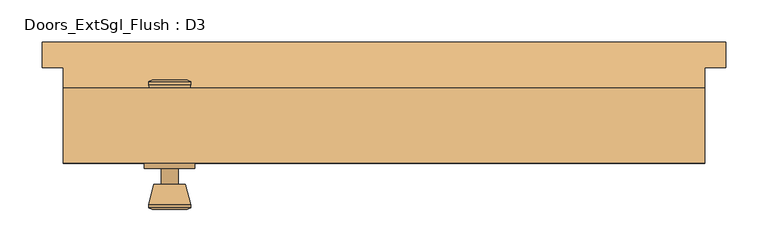
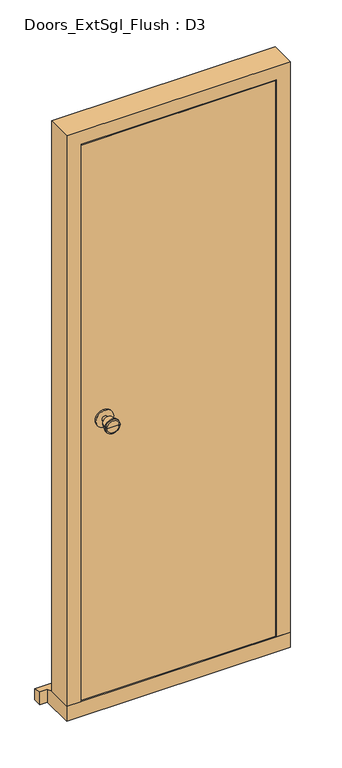
"""IFC4 building model written with IfcOpenShell, lengths in millimetres: door geometry, Doors_ExtSgl_Flush : D3."""

from ifc_helpers import new_model, si_unit, point, frame, frame_2d, origin, place, context, project, spatial, polyline, circle_curve, trimmed, segment, composite_curve, outline, extrude, faceted_brep, source, transform, mapped, element, save
from ifc_brep_helpers import plane_surface, cylinder_surface, revolved_surface, advanced_brep


def doors_extsgl_flush_d3_fcdd24de(model_context):
    return source(origin(), model_context, "Body", "SolidModel", [
        advanced_brep(
        [(-254.5, -85.1004, 1050.0), (-244.5, -85.1004, 1050.0), (-264.5, -85.1004, 1050.0), (-234.0241324, -134.1004, 1050.0), (-254.5, -134.1004, 1050.0), (-274.9758676, -134.1004, 1050.0), (-229.5, -132.2725319, 1050.0), (-279.5, -132.2725319, 1050.0), (-229.5, -128.8088537, 1050.0), (-279.5, -128.8088537, 1050.0), (-235.863764, -104.1004, 1050.0), (-273.136236, -104.1004, 1050.0), (-244.5, -104.1004, 1050.0), (-264.5, -104.1004, 1050.0)],
        [
            (0, 1),
            (1, 2, circle_curve(frame((-254.5, -85.1004, 1050.0), z_axis=(0.0, 1.0, 0.0), x_axis=(-1.0, 0.0, 0.0)), 10.0)),
            (2, 0),
            (2, 1, circle_curve(frame((-254.5, -85.1004, 1050.0), z_axis=(0.0, 1.0, 0.0), x_axis=(-1.0, 0.0, 0.0)), 10.0)),
            (3, 4),
            (4, 5),
            (5, 3, circle_curve(frame((-254.5, -134.1004, 1050.0), z_axis=(0.0, -1.0, 0.0), x_axis=(-1.0, 0.0, 0.0)), 20.4758676)),
            (3, 5, circle_curve(frame((-254.5, -134.1004, 1050.0), z_axis=(0.0, -1.0, 0.0), x_axis=(-1.0, 0.0, 0.0)), 20.4758676)),
            (6, 3),
            (5, 7),
            (7, 6, circle_curve(frame((-254.5, -132.2725319, 1050.0), z_axis=(0.0, -1.0, 0.0), x_axis=(-1.0, 0.0, 0.0)), 25.0)),
            (6, 7, circle_curve(frame((-254.5, -132.2725319, 1050.0), z_axis=(0.0, -1.0, 0.0), x_axis=(-1.0, 0.0, 0.0)), 25.0)),
            (8, 6),
            (7, 9),
            (9, 8, circle_curve(frame((-254.5, -128.8088537, 1050.0), z_axis=(0.0, -1.0, 0.0), x_axis=(-1.0, 0.0, 0.0)), 25.0)),
            (8, 9, circle_curve(frame((-254.5, -128.8088537, 1050.0), z_axis=(0.0, -1.0, 0.0), x_axis=(-1.0, 0.0, 0.0)), 25.0)),
            (10, 8),
            (9, 11),
            (11, 10, circle_curve(frame((-254.5, -104.1004, 1050.0), z_axis=(0.0, -1.0, 0.0), x_axis=(-1.0, 0.0, 0.0)), 18.636236)),
            (10, 11, circle_curve(frame((-254.5, -104.1004, 1050.0), z_axis=(0.0, -1.0, 0.0), x_axis=(-1.0, 0.0, 0.0)), 18.636236)),
            (12, 10),
            (11, 13),
            (13, 12, circle_curve(frame((-254.5, -104.1004, 1050.0), z_axis=(0.0, -1.0, 0.0), x_axis=(-1.0, 0.0, 0.0)), 10.0)),
            (12, 13, circle_curve(frame((-254.5, -104.1004, 1050.0), z_axis=(0.0, -1.0, 0.0), x_axis=(-1.0, 0.0, 0.0)), 10.0)),
            (1, 12),
            (13, 2),
        ],
        [
            plane_surface(frame((-254.5, -85.1004, 1050.0), z_axis=(0.0, 1.0, 0.0), x_axis=(-1.0, 0.0, 0.0))),
            plane_surface(frame((-254.5, -134.1004, 1050.0), z_axis=(0.0, -1.0, 0.0), x_axis=(-1.0, 0.0, 0.0))),
            revolved_surface(polyline([(-274.9758676, -134.1004, 1050.0), (-279.5, -132.2725319, 1050.0)]), (-254.5, -85.1004, 1050.0), (0.0, 1.0, 0.0)),
            cylinder_surface(frame((-254.5, -85.1004, 1050.0), z_axis=(0.0, 1.0, 0.0), x_axis=(-1.0, 0.0, 0.0)), 25.0),
            revolved_surface(polyline([(-279.5, -128.8088537, 1050.0), (-273.136236, -104.1004, 1050.0)]), (-254.5, -85.1004, 1050.0), (0.0, 1.0, 0.0)),
            plane_surface(frame((-254.5, -104.1004, 1050.0), z_axis=(0.0, 1.0, 0.0), x_axis=(-1.0, 0.0, 0.0))),
            cylinder_surface(frame((-254.5, -85.1004, 1050.0), z_axis=(0.0, 1.0, 0.0), x_axis=(-1.0, 0.0, 0.0)), 10.0),
        ],
        [
            (0, [[1, 2, 3]]),
            (0, [[-3, 4, -1]]),
            (1, [[5, 6, 7]]),
            (1, [[-6, -5, 8]]),
            (2, [[9, -7, 10, 11]]),
            (2, [[-10, -8, -9, 12]]),
            (3, [[13, -11, 14, 15]]),
            (3, [[-14, -12, -13, 16]]),
            (4, [[17, -15, 18, 19]]),
            (4, [[-18, -16, -17, 20]]),
            (5, [[21, -19, 22, 23]]),
            (5, [[-22, -20, -21, 24]]),
            (6, [[25, -23, 26, -2]]),
            (6, [[-26, -24, -25, -4]]),
        ],
    ),
        extrude(outline(composite_curve([segment(trimmed(circle_curve(frame_2d((1050.0, -254.5)), 30.0), [point((1050.0, -284.5))], [point((1050.0, -224.5))], False, "CARTESIAN"), True, "CONTINUOUS"), segment(trimmed(circle_curve(frame_2d((1050.0, -254.5)), 30.0), [point((1050.0, -224.5))], [point((1050.0, -284.5))], False, "CARTESIAN"), True, "CONTINUOUS")], self_intersect=False)), frame((0.0, -85.1004, 0.0), z_axis=(0.0, 1.0, 0.0), x_axis=(0.0, 0.0, 1.0)), (0.0, 0.0, 1.0), 6.0),
        advanced_brep(
        [(-254.5, -29.1004, 1050.0), (-264.5, -29.1004, 1050.0), (-244.5, -29.1004, 1050.0), (-234.0241324, 19.8996, 1050.0), (-274.9758676, 19.8996, 1050.0), (-254.5, 19.8996, 1050.0), (-229.5, 18.0717319, 1050.0), (-279.5, 18.0717319, 1050.0), (-229.5, 14.6080537, 1050.0), (-279.5, 14.6080537, 1050.0), (-235.863764, -10.1004, 1050.0), (-273.136236, -10.1004, 1050.0), (-244.5, -10.1004, 1050.0), (-264.5, -10.1004, 1050.0)],
        [
            (0, 1),
            (1, 2, circle_curve(frame((-254.5, -29.1004, 1050.0), z_axis=(0.0, -1.0, 0.0), x_axis=(-1.0, 0.0, 0.0)), 10.0)),
            (2, 0),
            (2, 1, circle_curve(frame((-254.5, -29.1004, 1050.0), z_axis=(0.0, -1.0, 0.0), x_axis=(-1.0, 0.0, 0.0)), 10.0)),
            (3, 4, circle_curve(frame((-254.5, 19.8996, 1050.0), z_axis=(0.0, 1.0, 0.0), x_axis=(-1.0, 0.0, 0.0)), 20.4758676)),
            (4, 5),
            (5, 3),
            (4, 3, circle_curve(frame((-254.5, 19.8996, 1050.0), z_axis=(0.0, 1.0, 0.0), x_axis=(-1.0, 0.0, 0.0)), 20.4758676)),
            (6, 7, circle_curve(frame((-254.5, 18.0717319, 1050.0), z_axis=(0.0, 1.0, 0.0), x_axis=(-1.0, 0.0, 0.0)), 25.0)),
            (7, 4),
            (3, 6),
            (7, 6, circle_curve(frame((-254.5, 18.0717319, 1050.0), z_axis=(0.0, 1.0, 0.0), x_axis=(-1.0, 0.0, 0.0)), 25.0)),
            (8, 9, circle_curve(frame((-254.5, 14.6080537, 1050.0), z_axis=(0.0, 1.0, 0.0), x_axis=(-1.0, 0.0, 0.0)), 25.0)),
            (9, 7),
            (6, 8),
            (9, 8, circle_curve(frame((-254.5, 14.6080537, 1050.0), z_axis=(0.0, 1.0, 0.0), x_axis=(-1.0, 0.0, 0.0)), 25.0)),
            (10, 11, circle_curve(frame((-254.5, -10.1004, 1050.0), z_axis=(0.0, 1.0, 0.0), x_axis=(-1.0, 0.0, 0.0)), 18.636236)),
            (11, 9),
            (8, 10),
            (11, 10, circle_curve(frame((-254.5, -10.1004, 1050.0), z_axis=(0.0, 1.0, 0.0), x_axis=(-1.0, 0.0, 0.0)), 18.636236)),
            (12, 13, circle_curve(frame((-254.5, -10.1004, 1050.0), z_axis=(0.0, 1.0, 0.0), x_axis=(-1.0, 0.0, 0.0)), 10.0)),
            (13, 11),
            (10, 12),
            (13, 12, circle_curve(frame((-254.5, -10.1004, 1050.0), z_axis=(0.0, 1.0, 0.0), x_axis=(-1.0, 0.0, 0.0)), 10.0)),
            (1, 13),
            (12, 2),
        ],
        [
            plane_surface(frame((-254.5, -29.1004, 1050.0), z_axis=(0.0, -1.0, 0.0), x_axis=(-1.0, 0.0, 0.0))),
            plane_surface(frame((-254.5, 19.8996, 1050.0), z_axis=(0.0, 1.0, 0.0), x_axis=(-1.0, 0.0, 0.0))),
            revolved_surface(polyline([(-274.9758676, 19.8996, 1050.0), (-279.5, 18.0717319, 1050.0)]), (-254.5, -29.1004, 1050.0), (0.0, -1.0, 0.0)),
            cylinder_surface(frame((-254.5, -29.1004, 1050.0), z_axis=(0.0, -1.0, 0.0), x_axis=(-1.0, 0.0, 0.0)), 25.0),
            revolved_surface(polyline([(-279.5, 14.6080537, 1050.0), (-273.136236, -10.1004, 1050.0)]), (-254.5, -29.1004, 1050.0), (0.0, -1.0, 0.0)),
            plane_surface(frame((-254.5, -10.1004, 1050.0), z_axis=(0.0, -1.0, 0.0), x_axis=(-1.0, 0.0, 0.0))),
            cylinder_surface(frame((-254.5, -29.1004, 1050.0), z_axis=(0.0, -1.0, 0.0), x_axis=(-1.0, 0.0, 0.0)), 10.0),
        ],
        [
            (0, [[1, 2, 3]]),
            (0, [[-3, 4, -1]]),
            (1, [[5, 6, 7]]),
            (1, [[8, -7, -6]]),
            (2, [[9, 10, -5, 11]]),
            (2, [[12, -11, -8, -10]]),
            (3, [[13, 14, -9, 15]]),
            (3, [[16, -15, -12, -14]]),
            (4, [[17, 18, -13, 19]]),
            (4, [[20, -19, -16, -18]]),
            (5, [[21, 22, -17, 23]]),
            (5, [[24, -23, -20, -22]]),
            (6, [[-2, 25, -21, 26]]),
            (6, [[-4, -26, -24, -25]]),
        ],
    ),
        extrude(outline(composite_curve([segment(trimmed(circle_curve(frame_2d((1050.0, -254.5)), 30.0), [point((1050.0, -284.5))], [point((1050.0, -224.5))], False, "CARTESIAN"), True, "CONTINUOUS"), segment(trimmed(circle_curve(frame_2d((1050.0, -254.5)), 30.0), [point((1050.0, -224.5))], [point((1050.0, -284.5))], False, "CARTESIAN"), True, "CONTINUOUS")], self_intersect=False)), frame((0.0, -35.1004, 0.0), z_axis=(0.0, 1.0, 0.0), x_axis=(0.0, 0.0, 1.0)), (0.0, 0.0, 1.0), 6.0),
        faceted_brep([(310.5, 9.8996, 54.5), (381.0, 9.8996, 54.5), (381.0, -79.1004, 54.5), (332.5, -79.1004, 54.5), (332.5, -32.1004, 54.5), (310.5, -32.1004, 54.5), (310.5, 9.8996, 2039.5), (-310.5, 9.8996, 2039.5), (-310.5, 9.8996, 54.5), (-381.0, 9.8996, 54.5), (-381.0, 9.8996, 2110.0), (381.0, 9.8996, 2110.0), (381.0, -79.1004, 2110.0), (-381.0, -79.1004, 2110.0), (-381.0, -79.1004, 54.5), (-332.5, -79.1004, 54.5), (-332.5, -79.1004, 2061.5), (332.5, -79.1004, 2061.5), (332.5, -32.1004, 2061.5), (-332.5, -32.1004, 2061.5), (-332.5, -32.1004, 54.5), (-310.5, -32.1004, 54.5), (-310.5, -32.1004, 2039.5), (310.5, -32.1004, 2039.5)], [[[0, 1, 2, 3, 4, 5]], [[1, 0, 6, 7, 8, 9, 10, 11]], [[2, 1, 11, 12]], [[3, 2, 12, 13, 14, 15, 16, 17]], [[4, 3, 17, 18]], [[5, 4, 18, 19, 20, 21, 22, 23]], [[0, 5, 23, 6]], [[7, 22, 21, 8]], [[8, 21, 20, 15, 14, 9]], [[13, 10, 9, 14]], [[19, 16, 15, 20]], [[12, 11, 10, 13]], [[18, 17, 16, 19]], [[6, 23, 22, 7]]]),
        extrude(outline(polyline([(329.5, -79.1004), (-330.4250294, -79.1004), (-330.4250294, -35.1004), (329.5, -35.1004), (329.5, -79.1004)])), frame((0.0, 0.0, 58.5), z_axis=(0.0, 0.0, 1.0), x_axis=(1.0, 0.0, 0.0)), (0.0, 0.0, 1.0), 2000.0),
        faceted_brep([(406.0, 64.8996, 0.0), (406.0, 64.8996, 38.5947221), (406.0, 34.8996, 47.2703282), (406.0, 34.8996, 0.0), (-406.0, 64.8996, 38.5947221), (-406.0, 64.8996, 0.0), (-406.0, 34.8996, 0.0), (-406.0, 34.8996, 47.2703282), (381.0, 34.8996, 0.0), (381.0, -79.1004, 0.0), (-381.0, -79.1004, 0.0), (-381.0, 34.8996, 0.0), (-381.0, 34.8996, 47.2703282), (-381.0, 9.8996, 54.5), (381.0, 9.8996, 54.5), (381.0, 34.8996, 47.2703282), (-381.0, -79.1004, 54.5), (381.0, -79.1004, 54.5)], [[[0, 1, 2, 3]], [[4, 5, 6, 7]], [[5, 0, 3, 8, 9, 10, 11, 6]], [[1, 0, 5, 4]], [[1, 4, 7, 12, 13, 14, 15, 2]], [[13, 16, 17, 14]], [[16, 10, 9, 17]], [[12, 11, 10, 16, 13]], [[11, 12, 7, 6]], [[8, 15, 14, 17, 9]], [[15, 8, 3, 2]]]),
    ])


if __name__ == "__main__":
    model = new_model("IFC4")
    model_context = context("Model", 3, world=origin())
    ifc_project = project(units=[si_unit("LENGTHUNIT", "METRE", prefix="MILLI")], contexts=[model_context])
    site = spatial("IfcSite", under=ifc_project)
    building = spatial("IfcBuilding", under=site)
    placement = place(None, origin())
    doors_extsgl_flush_d3_shape = doors_extsgl_flush_d3_fcdd24de(model_context)
    element("IfcDoor", 1, ObjectType="Doors_ExtSgl_Flush : D3", at=placement, inside=building, context=model_context, shape_type="MappedRepresentation", body=[
        mapped(doors_extsgl_flush_d3_shape, transform((0.0, 0.0, 0.0), x_axis=(1.0, 0.0, 0.0), y_axis=(0.0, 1.0, 0.0), z_axis=(0.0, 0.0, 1.0))),
    ])
    save(model, "model.ifc")

# Revit data of these elements
# Type "Doors_ExtSgl_Flush : D3"
#   Type Mark = "51"
#   Type Comments = "External Single"
#   Operation = "SingleSwingRight"
#   Construction Type Id = "MDOOR"
#   Keynote = "L20"
#   Analytic Construction = "Metal"
#   Wrap Layers (Int) from Ext = 177.5 mm
#   Wrap Layers (Ext) from Ext = 102.5 mm
#   Thickness = 44 mm
#   Rough Width = 762 mm
#   Rough Height = 2110 mm
#   O/A Frame Width = 64 mm
#   Heat Transfer Coefficient (U) = 3.7021 W/(m²·K)
#   Handle Z Distance = 1050 mm
#   FrameWidth = 42 mm
#   FrameOffset - External = 25 mm
#   FrameDepth = 89 mm
#   Door Panel Width = 659 mm
#   Door Panel Thickness = 44 mm
#   Door Panel Height = 2000 mm
#   Cill Thickness = 54.5 mm
#   Cill Projection = 30 mm
#   Handle X Distance = 75 mm
#   Height = 2110 mm
#   Structural Tolerance = 6.5 mm
#   Tolerance = 3 mm
#   Undercut = 4 mm
#   Width = 762 mm
#   Cill Extension = 25 mm
#   Cavity Closer Width = 50 mm
#   Cavity Closer Offset from Ext = 102.5 mm
#   Cavity Closer Depth = 85 mm
#   Vis - Ironmongery = yes
#   Vis - Cavity Closers = yes
#   Define Thermal Properties by = 1
#   Function = 1
#   Material Door = Door - Panel
#   Material Frame = Door - Frame/Mullion
#   Material Ironmongery = Door - Handle
#   Visual Light Transmittance = 0
#   Solar Heat Gain Coefficient = 0
#   Wall Closure = (empty or 0)
# Element 1 (IfcDoor, "Doors_ExtSgl_Flush : D3")
#   Materials on its faces: "Door - Handle", "Door - Frame/Mullion", "Door - Panel"
# Materials
#   "Door - Panel": class "Wood", colour RGB 210 159 95, transparency 0, Keynote = "L20", Cost = 0
#   "Door - Frame/Mullion": class "Wood", colour RGB 212 179 113, transparency 0, Keynote = "L20", Cost = 0
#   "Door - Handle": colour RGB 0 0 0, transparency 0, Keynote = "P21", Cost = 0
